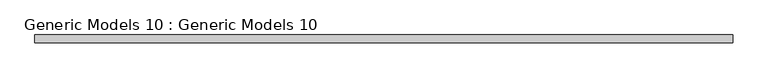
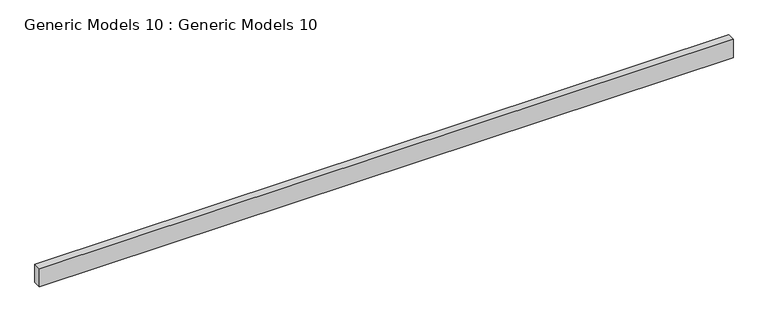
"""IFC4 building model written with IfcOpenShell, lengths in millimetres: proxy geometry, Generic Models 10 : Generic Models 10."""

from ifc_helpers import new_model, si_unit, frame, origin, place, context, project, spatial, polyline, outline, extrude, source, transform, mapped, element, save


def generic_models_10_generic_models_10_516a4994(model_context):
    return source(origin(), model_context, "Body", "SweptSolid", [
        extrude(outline(polyline([(12604.4370151, -3682.5004242), (12604.4370151, -3927.8342514), (-8934.7629849, -3927.8342514), (-8934.7629849, -3682.5004242), (12604.4370151, -3682.5004242)])), frame((0.0, 0.0, 25664.9816542), z_axis=(0.0, 0.0, 1.0), x_axis=(1.0, 0.0, 0.0)), (0.0, 0.0, 1.0), 596.7654914),
    ])


if __name__ == "__main__":
    model = new_model("IFC4")
    model_context = context("Model", 3, world=origin())
    ifc_project = project(units=[si_unit("LENGTHUNIT", "METRE", prefix="MILLI")], contexts=[model_context])
    site = spatial("IfcSite", under=ifc_project)
    building = spatial("IfcBuilding", under=site)
    placement = place(None, origin())
    generic_models_10_generic_models_10_shape = generic_models_10_generic_models_10_516a4994(model_context)
    element("IfcBuildingElementProxy", 1, Name="Generic Models 10 : Generic Models 10", ObjectType="Generic Models 10 : Generic Models 10", at=placement, inside=building, context=model_context, shape_type="MappedRepresentation", body=[
        mapped(generic_models_10_generic_models_10_shape, transform((0.0, 0.0, 0.0), x_axis=(1.0, 0.0, 0.0), y_axis=(0.0, 1.0, 0.0), z_axis=(0.0, 0.0, 1.0))),
    ])
    save(model, "model.ifc")
